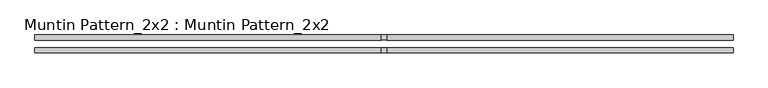
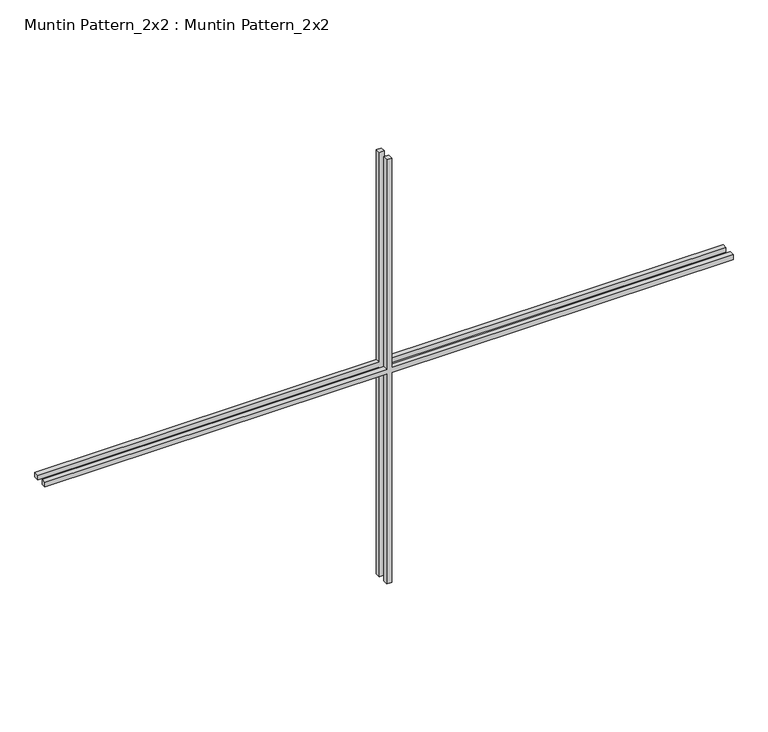
"""IFC4 building model written with IfcOpenShell, lengths in millimetres: proxy geometry, Muntin Pattern_2x2 : Muntin Pattern_2x2."""

from ifc_helpers import new_model, si_unit, frame, origin, place, context, project, spatial, polyline, outline, extrude, source, transform, mapped, element, save


def muntin_pattern_2x2_muntin_pattern_2x2_2dc59915(model_context):
    return source(origin(), model_context, "Body", "SweptSolid", [
        extrude(outline(polyline([(577.85, -6.35), (577.85, -876.3), (565.15, -876.3), (565.15, -6.35), (0.0, -6.35), (0.0, 6.35), (565.15, 6.35), (565.15, 876.3), (577.85, 876.3), (577.85, 6.35), (1143.0, 6.35), (1143.0, -6.35), (577.85, -6.35)])), frame((0.0, -22.225, 0.0), z_axis=(0.0, 1.0, 0.0), x_axis=(0.0, 0.0, 1.0)), (0.0, 0.0, 1.0), 12.7),
        extrude(outline(polyline([(577.85, -6.35), (577.85, -876.3), (565.15, -876.3), (565.15, -6.35), (0.0, -6.35), (0.0, 6.35), (565.15, 6.35), (565.15, 876.3), (577.85, 876.3), (577.85, 6.35), (1143.0, 6.35), (1143.0, -6.35), (577.85, -6.35)])), frame((0.0, 9.525, 0.0), z_axis=(0.0, 1.0, 0.0), x_axis=(0.0, 0.0, 1.0)), (0.0, 0.0, 1.0), 12.7),
    ])


if __name__ == "__main__":
    model = new_model("IFC4")
    model_context = context("Model", 3, world=origin())
    ifc_project = project(units=[si_unit("LENGTHUNIT", "METRE", prefix="MILLI")], contexts=[model_context])
    site = spatial("IfcSite", under=ifc_project)
    building = spatial("IfcBuilding", under=site)
    placement = place(None, origin())
    muntin_pattern_2x2_muntin_pattern_2x2_shape = muntin_pattern_2x2_muntin_pattern_2x2_2dc59915(model_context)
    element("IfcBuildingElementProxy", 1, Name="Muntin Pattern_2x2 : Muntin Pattern_2x2", ObjectType="Muntin Pattern_2x2 : Muntin Pattern_2x2", at=placement, inside=building, context=model_context, shape_type="MappedRepresentation", body=[
        mapped(muntin_pattern_2x2_muntin_pattern_2x2_shape, transform((0.0, 0.0, 0.0), x_axis=(1.0, 0.0, 0.0), y_axis=(0.0, 1.0, 0.0), z_axis=(0.0, 0.0, 1.0))),
    ])
    save(model, "model.ifc")

# Revit data of these elements
# Type "Muntin Pattern_2x2 : Muntin Pattern_2x2"
#   Width [instance default] = 4' - 0"
#   Thickness = 0' - 0 1/2"
#   Height [instance default] = 4' - 0"
#   Distance = 0' - 0 3/4"
#   Interior Material [instance default] = none
#   Exterior Material [instance default] = none
#   Default Elevation = 0
# Element 1 (IfcBuildingElementProxy, "Muntin Pattern_2x2 : Muntin Pattern_2x2")
#   Width = 5' - 9"
#   Height = 3' - 9"
#   Interior Material = Wood - Stained
#   Exterior Material = Clad - White
#   Materials on its faces: "Clad - White", "Wood - Stained"
# Materials
#   "Clad - White": class "Wood", colour RGB 242 242 238, transparency 0, Cost = 0
#   "Wood - Stained": class "Wood", colour RGB 224 178 126, transparency 0, Cost = 0
